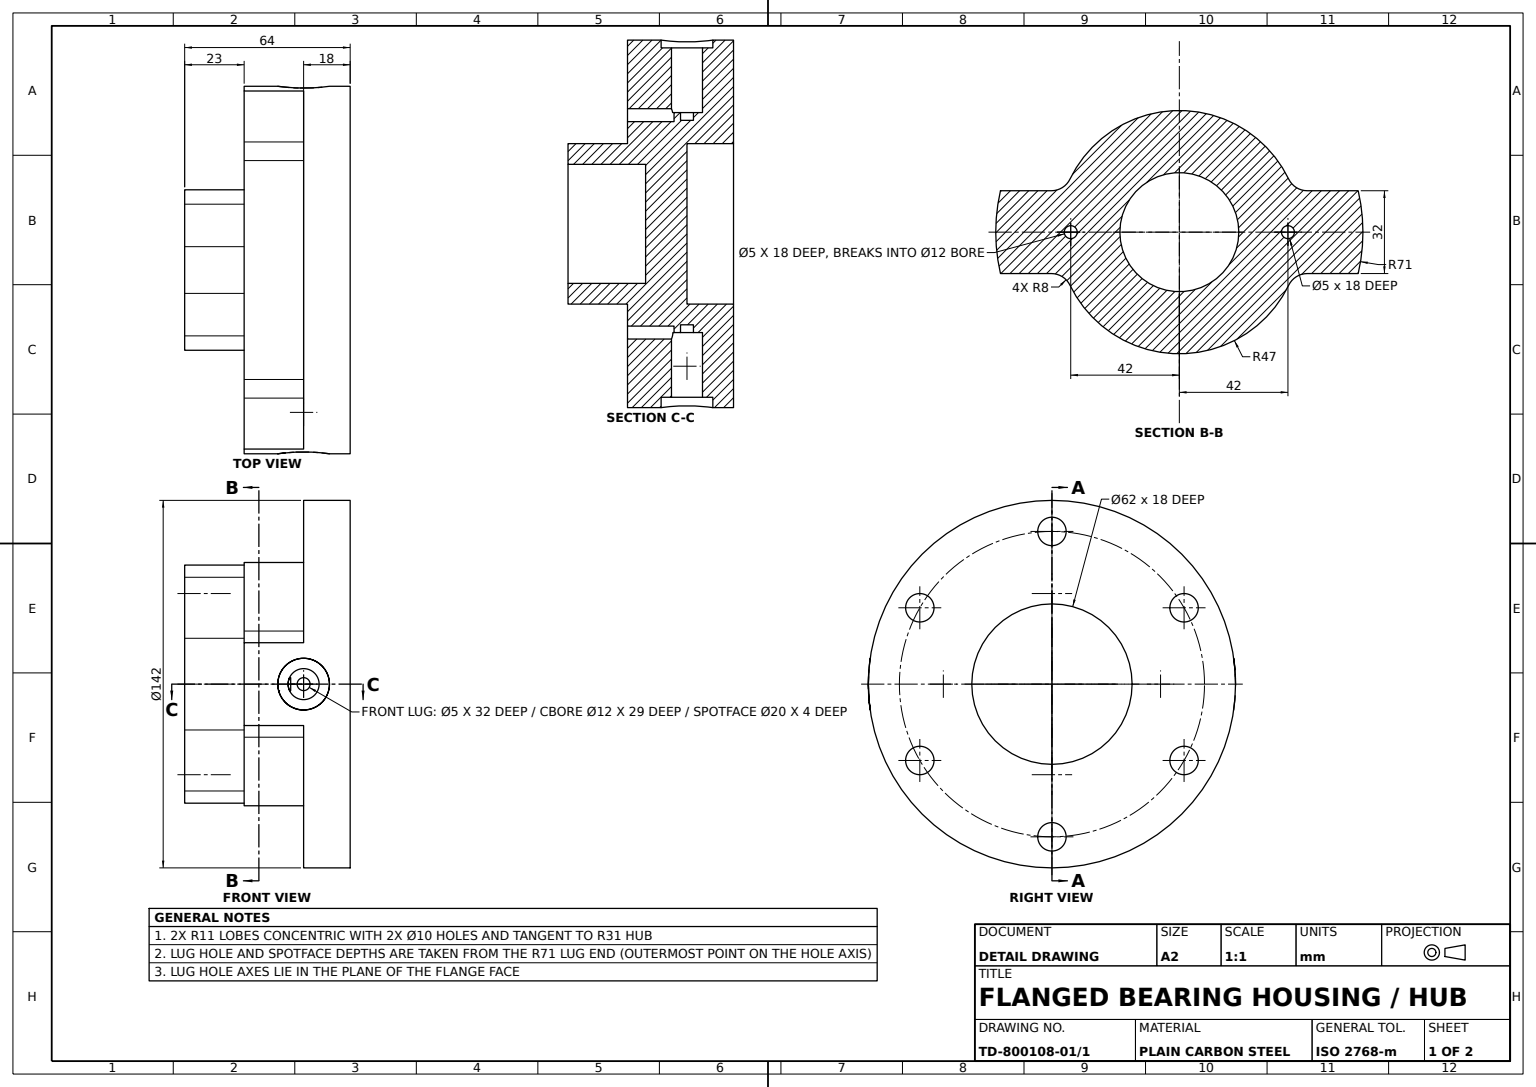
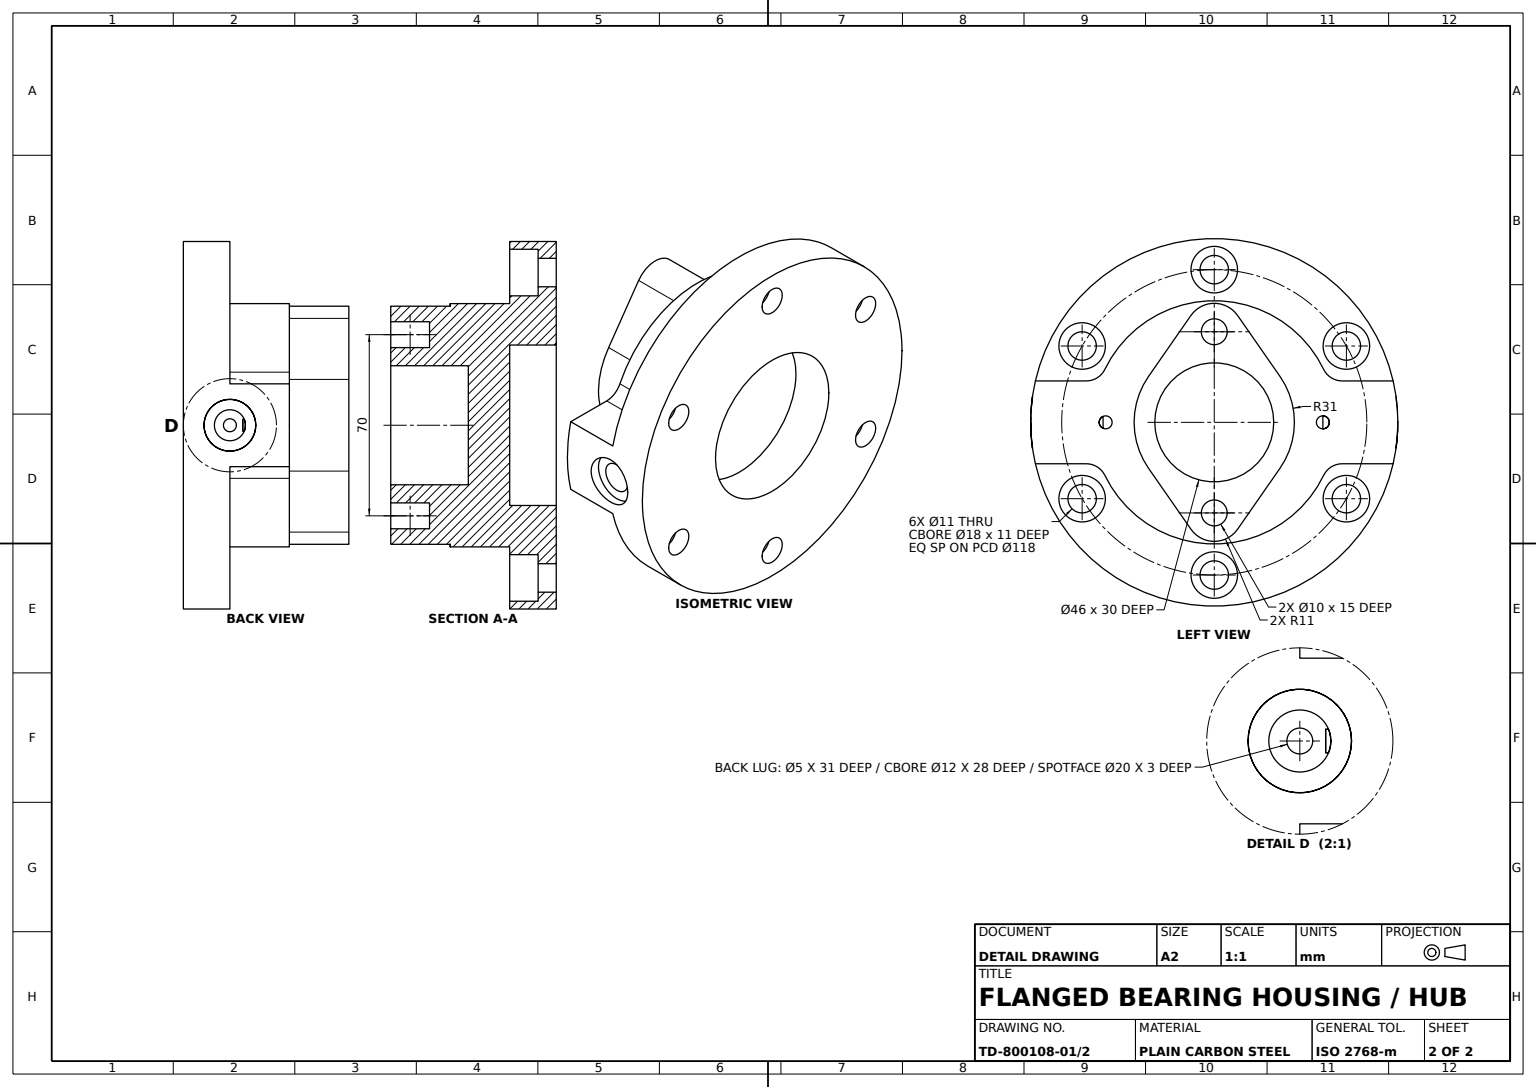
from build123d import *
from build123d.topology import SkipClean

# Parameters (mm, degrees)
FLANGE_SKETCH_R              = 71
FLANGE_142_DEPTH             = 18
BODY_BOSS_WITH_LUGS_DEPTH    = 23
FLANGE_COUNTERBORE_SKETCH_R  = 9
FLANGE_COUNTERBORES_6X_DEPTH = 11
FLANGE_HOLE_SKETCH_R         = 5.5
FLANGE_HOLES_6X_11_DEPTH     = 20
TOP_BOSS_DEPTH               = 23
BORE_SKETCH_R                = 23
BORE_46_DEPTH                = 30
TOP_BOSS_HOLE_SKETCH_R       = 5
TOP_BOSS_HOLES_DEPTH         = 15
THROUGH_BORE_SKETCH_R        = 31
THROUGH_BORE_62_DEPTH        = 18
BODY_BOSS_HOLE_SKETCH_R      = 2.5
BODY_BOSS_HOLES_DEPTH        = 18
LUG_A_SPOT_FACE_DEPTH        = 4
LUG_A_HOLE_12_SKETCH_R       = 6
LUG_A_HOLE_12_DEPTH          = 25
LUG_A_HOLE_5_SKETCH_R        = 2.5
LUG_A_HOLE_5_DEPTH           = 3
LUG_START                    = 4
LUG_B_SPOT_FACE_SKETCH_R     = 10
LUG_B_SPOT_FACE_DEPTH        = 4
LUG_START_2                  = -25
LUG_B_HOLE_12_SKETCH_R       = 6
LUG_B_HOLE_12_DEPTH          = 25
LUG_START_3                  = -3
LUG_B_HOLE_5_SKETCH_R        = 2.5
LUG_B_HOLE_5_DEPTH           = 3


with BuildPart() as part:
    # Flange Sketch → Flange Ø142 (new body)
    with BuildSketch(Plane.XY):
        Circle(FLANGE_SKETCH_R)
    extrude(amount=FLANGE_142_DEPTH)

    # Body Boss Sketch → Body Boss With Lugs (add)
    with SkipClean():  # the faces are left unmerged after this step: merging them gives an invalid solid
        with BuildSketch(Plane.XY.offset(18)):
            with BuildLine():
                Line((-69.173694422, 16), (-49.487372127, 16))
                ThreePointArc((-49.487372127, 16), (-45.240448106, 17.22035131), (-42.289208908, 20.509090909))
                ThreePointArc((-42.289208908, 20.509090909), (0, 47), (42.289208908, 20.509090909))
                ThreePointArc((42.289208908, 20.509090909), (45.240448106, 17.22035131), (49.487372127, 16))
                Line((49.487372127, 16), (69.173694422, 16))
                ThreePointArc((69.173694422, 16), (71, 0), (69.173694422, -16))
                Line((69.173694422, -16), (49.487372127, -16))
                ThreePointArc((49.487372127, -16), (45.240448106, -17.22035131), (42.289208908, -20.509090909))
                ThreePointArc((42.289208908, -20.509090909), (0, -47), (-42.289208908, -20.509090909))
                ThreePointArc((-42.289208908, -20.509090909), (-45.240448106, -17.22035131), (-49.487372127, -16))
                Line((-49.487372127, -16), (-69.173694422, -16))
                ThreePointArc((-69.173694422, -16), (-71, 0), (-69.173694422, 16))
            make_face()
        extrude(amount=BODY_BOSS_WITH_LUGS_DEPTH)

    # Flange Counterbore Sketch → Flange Counterbores 6x (cut)
    with SkipClean():  # the faces are left unmerged after this step: merging them gives an invalid solid
        with BuildSketch(Plane.XY.offset(18)):
            with Locations((0, 59)):
                Circle(FLANGE_COUNTERBORE_SKETCH_R)
            with Locations((51.095498823, 29.5)):
                Circle(FLANGE_COUNTERBORE_SKETCH_R)
            with Locations((51.095498823, -29.5)):
                Circle(FLANGE_COUNTERBORE_SKETCH_R)
            with Locations((0, -59)):
                Circle(FLANGE_COUNTERBORE_SKETCH_R)
            with Locations((-51.095498823, -29.5)):
                Circle(FLANGE_COUNTERBORE_SKETCH_R)
            with Locations((-51.095498823, 29.5)):
                Circle(FLANGE_COUNTERBORE_SKETCH_R)
        extrude(amount=-FLANGE_COUNTERBORES_6X_DEPTH, mode=Mode.SUBTRACT)

    # Flange Hole Sketch → Flange Holes 6xØ11 (cut)
    with SkipClean():  # the faces are left unmerged after this step: merging them gives an invalid solid
        with BuildSketch(Plane.XY.offset(18)):
            with Locations((0, 59)):
                Circle(FLANGE_HOLE_SKETCH_R)
            with Locations((51.095498823, 29.5)):
                Circle(FLANGE_HOLE_SKETCH_R)
            with Locations((51.095498823, -29.5)):
                Circle(FLANGE_HOLE_SKETCH_R)
            with Locations((0, -59)):
                Circle(FLANGE_HOLE_SKETCH_R)
            with Locations((-51.095498823, -29.5)):
                Circle(FLANGE_HOLE_SKETCH_R)
            with Locations((-51.095498823, 29.5)):
                Circle(FLANGE_HOLE_SKETCH_R)
        extrude(amount=-FLANGE_HOLES_6X_11_DEPTH, mode=Mode.SUBTRACT)

    # Top Boss Sketch → Top Boss (add)
    with SkipClean():  # the faces are left unmerged after this step: merging them gives an invalid solid
        with BuildSketch(Plane.XY.offset(41)):
            with BuildLine():
                Line((9.027169873, -41.285714286), (25.440206006, -17.714285714))
                ThreePointArc((25.440206006, -17.714285714), (31, 0), (25.440206006, 17.714285714))
                Line((25.440206006, 17.714285714), (9.027169873, 41.285714286))
                ThreePointArc((9.027169873, 41.285714286), (0, 46), (-9.027169873, 41.285714286))
                Line((-9.027169873, 41.285714286), (-25.440206006, 17.714285714))
                ThreePointArc((-25.440206006, 17.714285714), (-31, 0), (-25.440206006, -17.714285714))
                Line((-25.440206006, -17.714285714), (-9.027169873, -41.285714286))
                ThreePointArc((-9.027169873, -41.285714286), (0, -46), (9.027169873, -41.285714286))
            make_face()
        extrude(amount=TOP_BOSS_DEPTH)

    # Bore Sketch → Bore Ø46 (cut)
    with SkipClean():  # the faces are left unmerged after this step: merging them gives an invalid solid
        with BuildSketch(Plane.XY.offset(64)):
            Circle(BORE_SKETCH_R)
        extrude(amount=-BORE_46_DEPTH, mode=Mode.SUBTRACT)

    # Top Boss Hole Sketch → Top Boss Holes (cut)
    with SkipClean():  # the faces are left unmerged after this step: merging them gives an invalid solid
        with BuildSketch(Plane.XY.offset(64)):
            with Locations((0, 35)):
                Circle(TOP_BOSS_HOLE_SKETCH_R)
            with Locations((0, -35)):
                Circle(TOP_BOSS_HOLE_SKETCH_R)
        extrude(amount=-TOP_BOSS_HOLES_DEPTH, mode=Mode.SUBTRACT)

    # Through Bore Sketch → Through Bore Ø62 (cut)
    with SkipClean():  # the faces are left unmerged after this step: merging them gives an invalid solid
        with BuildSketch(Plane(origin=(0, 0, 0), x_dir=(-1, 0, 0), z_dir=(0, 0, -1))):
            Circle(THROUGH_BORE_SKETCH_R)
        extrude(amount=-THROUGH_BORE_62_DEPTH, mode=Mode.SUBTRACT)

    # Body Boss Hole Sketch → Body Boss Holes (cut)
    with SkipClean():  # the faces are left unmerged after this step: merging them gives an invalid solid
        with BuildSketch(Plane.XY.offset(41)):
            with Locations((-42, 0)):
                Circle(BODY_BOSS_HOLE_SKETCH_R)
            with Locations((42, 0)):
                Circle(BODY_BOSS_HOLE_SKETCH_R)
        extrude(amount=-BODY_BOSS_HOLES_DEPTH, mode=Mode.SUBTRACT)

    # Lug A Spot Face Sketch → Lug A Spot Face (cut)
    with SkipClean():  # the faces are left unmerged after this step: merging them gives an invalid solid
        with BuildSketch(Plane(origin=(72, 0, 0), x_dir=(0, 0, -1), z_dir=(1, 0, 0))):
            with BuildLine():
                ThreePointArc((-8, 0), (-10.928932188, 7.071067812), (-18, 10))
                Line((-18, 10), (-18, -10))
                ThreePointArc((-18, -10), (-10.928932188, -7.071067812), (-8, 0))
            make_face()
            with BuildLine():
                Line((-18, -10), (-18, 10))
                ThreePointArc((-18, 10), (-28, 0), (-18, -10))
            make_face()
        extrude(amount=-LUG_A_SPOT_FACE_DEPTH, mode=Mode.SUBTRACT)

    # Lug A Hole Ø12 Sketch → Lug A Hole Ø12 (cut)
    with SkipClean():  # the faces are left unmerged after this step: merging them gives an invalid solid
        with BuildSketch(Plane(origin=(68, 0, 0), x_dir=(0, 0, -1), z_dir=(1, 0, 0))):
            with Locations((-18, 0)):
                Circle(LUG_A_HOLE_12_SKETCH_R)
        extrude(amount=-LUG_A_HOLE_12_DEPTH, mode=Mode.SUBTRACT)

    # Lug A Hole Ø5 Sketch → Lug A Hole Ø5 (cut)
    with SkipClean():  # the faces are left unmerged after this step: merging them gives an invalid solid
        with BuildSketch(Plane(origin=(43, 0, 0), x_dir=(0, 0, -1), z_dir=(1, 0, 0))):
            with Locations((-18, 0)):
                Circle(LUG_A_HOLE_5_SKETCH_R)
        extrude(amount=-LUG_A_HOLE_5_DEPTH, mode=Mode.SUBTRACT)

    # Lug B Spot Face Sketch → Lug B Spot Face (cut)
    with SkipClean():  # the faces are left unmerged after this step: merging them gives an invalid solid
        with BuildSketch(Plane(origin=(-71, 0, 0), x_dir=(0, 0, -1), z_dir=(1, 0, 0)).offset(LUG_START)):
            with Locations((-18, 0)):
                Circle(LUG_B_SPOT_FACE_SKETCH_R)
        extrude(amount=-LUG_B_SPOT_FACE_DEPTH, mode=Mode.SUBTRACT)

    # Lug B Hole Ø12 Sketch → Lug B Hole Ø12 (cut)
    with SkipClean():  # the faces are left unmerged after this step: merging them gives an invalid solid
        with BuildSketch(Plane.ZY.offset(67).offset(LUG_START_2)):
            with Locations(Location((18, 0, 0), (0, 0, 180))):
                Circle(LUG_B_HOLE_12_SKETCH_R)
        extrude(amount=LUG_B_HOLE_12_DEPTH, mode=Mode.SUBTRACT)

    # Lug B Hole Ø5 Sketch → Lug B Hole Ø5 (cut)
    with SkipClean():  # the faces are left unmerged after this step: merging them gives an invalid solid
        with BuildSketch(Plane.ZY.offset(42).offset(LUG_START_3)):
            with Locations(Location((18, 0, 0), (0, 0, 180))):
                Circle(LUG_B_HOLE_5_SKETCH_R)
        extrude(amount=LUG_B_HOLE_5_DEPTH, mode=Mode.SUBTRACT)


solid = part.part
